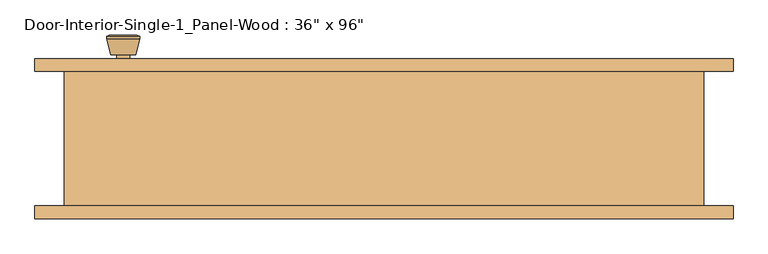
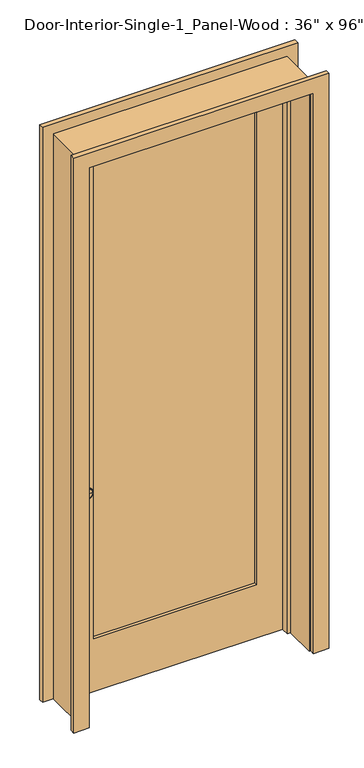
"""IFC4 building model written with IfcOpenShell, lengths in millimetres: door geometry."""

from ifc_helpers import new_model, si_unit, point, frame, frame_2d, origin, place, context, project, spatial, polyline, circle_curve, trimmed, segment, composite_curve, outline, extrude, faceted_brep, source, transform, mapped, element, save
from ifc_brep_helpers import plane_surface, cylinder_surface, revolved_surface, advanced_brep


def door_8805718f(model_context):
    return source(origin(), model_context, "Body", "SolidModel", [
        advanced_brep(
        [(-393.7, 57.5, 914.4), (-383.7, 57.5, 914.4), (-403.7, 57.5, 914.4), (-373.2241324, 8.5, 914.4), (-393.7, 8.5, 914.4), (-414.1758676, 8.5, 914.4), (-368.7, 10.3278681, 914.4), (-418.7, 10.3278681, 914.4), (-368.7, 13.7915463, 914.4), (-418.7, 13.7915463, 914.4), (-375.063764, 38.5, 914.4), (-412.336236, 38.5, 914.4), (-383.7, 38.5, 914.4), (-403.7, 38.5, 914.4)],
        [
            (0, 1),
            (1, 2, circle_curve(frame((-393.7, 57.5, 914.4), z_axis=(0.0, 1.0, 0.0), x_axis=(-1.0, 0.0, 0.0)), 10.0)),
            (2, 0),
            (2, 1, circle_curve(frame((-393.7, 57.5, 914.4), z_axis=(0.0, 1.0, 0.0), x_axis=(-1.0, 0.0, 0.0)), 10.0)),
            (3, 4),
            (4, 5),
            (5, 3, circle_curve(frame((-393.7, 8.5, 914.4), z_axis=(0.0, -1.0, 0.0), x_axis=(-1.0, 0.0, 0.0)), 20.4758676)),
            (3, 5, circle_curve(frame((-393.7, 8.5, 914.4), z_axis=(0.0, -1.0, 0.0), x_axis=(-1.0, 0.0, 0.0)), 20.4758676)),
            (6, 3),
            (5, 7),
            (7, 6, circle_curve(frame((-393.7, 10.3278681, 914.4), z_axis=(0.0, -1.0, 0.0), x_axis=(-1.0, 0.0, 0.0)), 25.0)),
            (6, 7, circle_curve(frame((-393.7, 10.3278681, 914.4), z_axis=(0.0, -1.0, 0.0), x_axis=(-1.0, 0.0, 0.0)), 25.0)),
            (8, 6),
            (7, 9),
            (9, 8, circle_curve(frame((-393.7, 13.7915463, 914.4), z_axis=(0.0, -1.0, 0.0), x_axis=(-1.0, 0.0, 0.0)), 25.0)),
            (8, 9, circle_curve(frame((-393.7, 13.7915463, 914.4), z_axis=(0.0, -1.0, 0.0), x_axis=(-1.0, 0.0, 0.0)), 25.0)),
            (10, 8),
            (9, 11),
            (11, 10, circle_curve(frame((-393.7, 38.5, 914.4), z_axis=(0.0, -1.0, 0.0), x_axis=(-1.0, 0.0, 0.0)), 18.636236)),
            (10, 11, circle_curve(frame((-393.7, 38.5, 914.4), z_axis=(0.0, -1.0, 0.0), x_axis=(-1.0, 0.0, 0.0)), 18.636236)),
            (12, 10),
            (11, 13),
            (13, 12, circle_curve(frame((-393.7, 38.5, 914.4), z_axis=(0.0, -1.0, 0.0), x_axis=(-1.0, 0.0, 0.0)), 10.0)),
            (12, 13, circle_curve(frame((-393.7, 38.5, 914.4), z_axis=(0.0, -1.0, 0.0), x_axis=(-1.0, 0.0, 0.0)), 10.0)),
            (1, 12),
            (13, 2),
        ],
        [
            plane_surface(frame((-393.7, 57.5, 914.4), z_axis=(0.0, 1.0, 0.0), x_axis=(-1.0, 0.0, 0.0))),
            plane_surface(frame((-393.7, 8.5, 914.4), z_axis=(0.0, -1.0, 0.0), x_axis=(-1.0, 0.0, 0.0))),
            revolved_surface(polyline([(-414.1758676, 8.5, 914.4), (-418.7, 10.3278681, 914.4)]), (-393.7, 57.5, 914.4), (0.0, 1.0, 0.0)),
            cylinder_surface(frame((-393.7, 57.5, 914.4), z_axis=(0.0, 1.0, 0.0), x_axis=(-1.0, 0.0, 0.0)), 25.0),
            revolved_surface(polyline([(-418.7, 13.7915463, 914.4), (-412.336236, 38.5, 914.4)]), (-393.7, 57.5, 914.4), (0.0, 1.0, 0.0)),
            plane_surface(frame((-393.7, 38.5, 914.4), z_axis=(0.0, 1.0, 0.0), x_axis=(-1.0, 0.0, 0.0))),
            cylinder_surface(frame((-393.7, 57.5, 914.4), z_axis=(0.0, 1.0, 0.0), x_axis=(-1.0, 0.0, 0.0)), 10.0),
        ],
        [
            (0, [[1, 2, 3]]),
            (0, [[-3, 4, -1]]),
            (1, [[5, 6, 7]]),
            (1, [[-6, -5, 8]]),
            (2, [[9, -7, 10, 11]]),
            (2, [[-10, -8, -9, 12]]),
            (3, [[13, -11, 14, 15]]),
            (3, [[-14, -12, -13, 16]]),
            (4, [[17, -15, 18, 19]]),
            (4, [[-18, -16, -17, 20]]),
            (5, [[21, -19, 22, 23]]),
            (5, [[-22, -20, -21, 24]]),
            (6, [[25, -23, 26, -2]]),
            (6, [[-26, -24, -25, -4]]),
        ],
    ),
        extrude(outline(composite_curve([segment(trimmed(circle_curve(frame_2d((914.4, -393.7)), 30.0), [point((914.4, -423.7))], [point((914.4, -363.7))], False, "CARTESIAN"), True, "CONTINUOUS"), segment(trimmed(circle_curve(frame_2d((914.4, -393.7)), 30.0), [point((914.4, -363.7))], [point((914.4, -423.7))], False, "CARTESIAN"), True, "CONTINUOUS")], self_intersect=False)), frame((0.0, 57.5, 0.0), z_axis=(0.0, 1.0, 0.0), x_axis=(0.0, 0.0, 1.0)), (0.0, 0.0, 1.0), 6.0),
        advanced_brep(
        [(-393.7, 104.425, 914.4), (-403.7, 104.425, 914.4), (-383.7, 104.425, 914.4), (-373.2241324, 153.425, 914.4), (-414.1758676, 153.425, 914.4), (-393.7, 153.425, 914.4), (-368.7, 151.5971319, 914.4), (-418.7, 151.5971319, 914.4), (-368.7, 148.1334537, 914.4), (-418.7, 148.1334537, 914.4), (-375.063764, 123.425, 914.4), (-412.336236, 123.425, 914.4), (-383.7, 123.425, 914.4), (-403.7, 123.425, 914.4)],
        [
            (0, 1),
            (1, 2, circle_curve(frame((-393.7, 104.425, 914.4), z_axis=(0.0, -1.0, 0.0), x_axis=(-1.0, 0.0, 0.0)), 10.0)),
            (2, 0),
            (2, 1, circle_curve(frame((-393.7, 104.425, 914.4), z_axis=(0.0, -1.0, 0.0), x_axis=(-1.0, 0.0, 0.0)), 10.0)),
            (3, 4, circle_curve(frame((-393.7, 153.425, 914.4), z_axis=(0.0, 1.0, 0.0), x_axis=(-1.0, 0.0, 0.0)), 20.4758676)),
            (4, 5),
            (5, 3),
            (4, 3, circle_curve(frame((-393.7, 153.425, 914.4), z_axis=(0.0, 1.0, 0.0), x_axis=(-1.0, 0.0, 0.0)), 20.4758676)),
            (6, 7, circle_curve(frame((-393.7, 151.5971319, 914.4), z_axis=(0.0, 1.0, 0.0), x_axis=(-1.0, 0.0, 0.0)), 25.0)),
            (7, 4),
            (3, 6),
            (7, 6, circle_curve(frame((-393.7, 151.5971319, 914.4), z_axis=(0.0, 1.0, 0.0), x_axis=(-1.0, 0.0, 0.0)), 25.0)),
            (8, 9, circle_curve(frame((-393.7, 148.1334537, 914.4), z_axis=(0.0, 1.0, 0.0), x_axis=(-1.0, 0.0, 0.0)), 25.0)),
            (9, 7),
            (6, 8),
            (9, 8, circle_curve(frame((-393.7, 148.1334537, 914.4), z_axis=(0.0, 1.0, 0.0), x_axis=(-1.0, 0.0, 0.0)), 25.0)),
            (10, 11, circle_curve(frame((-393.7, 123.425, 914.4), z_axis=(0.0, 1.0, 0.0), x_axis=(-1.0, 0.0, 0.0)), 18.636236)),
            (11, 9),
            (8, 10),
            (11, 10, circle_curve(frame((-393.7, 123.425, 914.4), z_axis=(0.0, 1.0, 0.0), x_axis=(-1.0, 0.0, 0.0)), 18.636236)),
            (12, 13, circle_curve(frame((-393.7, 123.425, 914.4), z_axis=(0.0, 1.0, 0.0), x_axis=(-1.0, 0.0, 0.0)), 10.0)),
            (13, 11),
            (10, 12),
            (13, 12, circle_curve(frame((-393.7, 123.425, 914.4), z_axis=(0.0, 1.0, 0.0), x_axis=(-1.0, 0.0, 0.0)), 10.0)),
            (1, 13),
            (12, 2),
        ],
        [
            plane_surface(frame((-393.7, 104.425, 914.4), z_axis=(0.0, -1.0, 0.0), x_axis=(-1.0, 0.0, 0.0))),
            plane_surface(frame((-393.7, 153.425, 914.4), z_axis=(0.0, 1.0, 0.0), x_axis=(-1.0, 0.0, 0.0))),
            revolved_surface(polyline([(-414.1758676, 153.425, 914.4), (-418.7, 151.5971319, 914.4)]), (-393.7, 104.425, 914.4), (0.0, -1.0, 0.0)),
            cylinder_surface(frame((-393.7, 104.425, 914.4), z_axis=(0.0, -1.0, 0.0), x_axis=(-1.0, 0.0, 0.0)), 25.0),
            revolved_surface(polyline([(-418.7, 148.1334537, 914.4), (-412.336236, 123.425, 914.4)]), (-393.7, 104.425, 914.4), (0.0, -1.0, 0.0)),
            plane_surface(frame((-393.7, 123.425, 914.4), z_axis=(0.0, -1.0, 0.0), x_axis=(-1.0, 0.0, 0.0))),
            cylinder_surface(frame((-393.7, 104.425, 914.4), z_axis=(0.0, -1.0, 0.0), x_axis=(-1.0, 0.0, 0.0)), 10.0),
        ],
        [
            (0, [[1, 2, 3]]),
            (0, [[-3, 4, -1]]),
            (1, [[5, 6, 7]]),
            (1, [[8, -7, -6]]),
            (2, [[9, 10, -5, 11]]),
            (2, [[12, -11, -8, -10]]),
            (3, [[13, 14, -9, 15]]),
            (3, [[16, -15, -12, -14]]),
            (4, [[17, 18, -13, 19]]),
            (4, [[20, -19, -16, -18]]),
            (5, [[21, 22, -17, 23]]),
            (5, [[24, -23, -20, -22]]),
            (6, [[-2, 25, -21, 26]]),
            (6, [[-4, -26, -24, -25]]),
        ],
    ),
        extrude(outline(composite_curve([segment(trimmed(circle_curve(frame_2d((914.4, -393.7)), 30.0), [point((914.4, -423.7))], [point((914.4, -363.7))], False, "CARTESIAN"), True, "CONTINUOUS"), segment(trimmed(circle_curve(frame_2d((914.4, -393.7)), 30.0), [point((914.4, -363.7))], [point((914.4, -423.7))], False, "CARTESIAN"), True, "CONTINUOUS")], self_intersect=False)), frame((0.0, 98.425, 0.0), z_axis=(0.0, 1.0, 0.0), x_axis=(0.0, 0.0, 1.0)), (0.0, 0.0, 1.0), 6.0),
        faceted_brep([(482.6, 98.425, 0.0), (482.6, -104.775, 0.0), (457.2, -104.775, 0.0), (457.2, 28.575, 0.0), (444.5, 28.575, 0.0), (444.5, 63.5, 0.0), (457.2, 63.5, 0.0), (457.2, 98.425, 0.0), (482.6, 98.425, 2463.8), (482.6, -104.775, 2463.8), (-482.6, -104.775, 2463.8), (-482.6, -104.775, 0.0), (-457.2, -104.775, 0.0), (-457.2, -104.775, 2438.4), (457.2, -104.775, 2438.4), (457.2, 28.575, 2438.4), (-457.2, 28.575, 2438.4), (-457.2, 28.575, 0.0), (-444.5, 28.575, 0.0), (-444.5, 28.575, 2425.7), (444.5, 28.575, 2425.7), (444.5, 63.5, 2425.7), (-444.5, 63.5, 2425.7), (-444.5, 63.5, 0.0), (-457.2, 63.5, 0.0), (-457.2, 63.5, 2438.4), (457.2, 63.5, 2438.4), (457.2, 98.425, 2438.4), (-457.2, 98.425, 2438.4), (-457.2, 98.425, 0.0), (-482.6, 98.425, 0.0), (-482.6, 98.425, 2463.8)], [[[0, 1, 2, 3, 4, 5, 6, 7]], [[1, 0, 8, 9]], [[2, 1, 9, 10, 11, 12, 13, 14]], [[3, 2, 14, 15]], [[4, 3, 15, 16, 17, 18, 19, 20]], [[5, 4, 20, 21]], [[6, 5, 21, 22, 23, 24, 25, 26]], [[7, 6, 26, 27]], [[0, 7, 27, 28, 29, 30, 31, 8]], [[9, 8, 31, 10]], [[15, 14, 13, 16]], [[21, 20, 19, 22]], [[27, 26, 25, 28]], [[30, 29, 24, 23, 18, 17, 12, 11]], [[10, 31, 30, 11]], [[16, 13, 12, 17]], [[22, 19, 18, 23]], [[28, 25, 24, 29]]]),
        extrude(outline(polyline([(2438.4, -457.2), (0.0, -457.2), (0.0, 457.2), (2438.4, 457.2), (2438.4, -457.2)]), holes=[polyline([(2319.3375, -336.55), (2319.3375, 336.55), (231.775, 336.55), (231.775, -336.55), (2319.3375, -336.55)])]), frame((0.0, 63.5, 0.0), z_axis=(0.0, 1.0, 0.0), x_axis=(0.0, 0.0, 1.0)), (0.0, 0.0, 1.0), 34.925),
        extrude(outline(polyline([(336.55, 75.1416667), (-336.55, 75.1416667), (-336.55, 86.7833333), (336.55, 86.7833333), (336.55, 75.1416667)])), frame((0.0, 0.0, 231.775), z_axis=(0.0, 0.0, 1.0), x_axis=(1.0, 0.0, 0.0)), (0.0, 0.0, 1.0), 2087.5625),
        extrude(outline(polyline([(0.0, 463.55), (0.0, 527.05), (2508.25, 527.05), (2508.25, -527.05), (0.0, -527.05), (0.0, -463.55), (2444.75, -463.55), (2444.75, 463.55), (0.0, 463.55)])), frame((0.0, 98.425, 0.0), z_axis=(0.0, 1.0, 0.0), x_axis=(0.0, 0.0, 1.0)), (0.0, 0.0, 1.0), 19.05),
        extrude(outline(polyline([(0.0, 463.55), (0.0, 527.05), (2508.25, 527.05), (2508.25, -527.05), (0.0, -527.05), (0.0, -463.55), (2444.75, -463.55), (2444.75, 463.55), (0.0, 463.55)])), frame((0.0, -123.825, 0.0), z_axis=(0.0, 1.0, 0.0), x_axis=(0.0, 0.0, 1.0)), (0.0, 0.0, 1.0), 19.05),
    ])


if __name__ == "__main__":
    model = new_model("IFC4")
    model_context = context("Model", 3, world=origin())
    ifc_project = project(units=[si_unit("LENGTHUNIT", "METRE", prefix="MILLI")], contexts=[model_context])
    site = spatial("IfcSite", under=ifc_project)
    building = spatial("IfcBuilding", under=site)
    placement = place(None, origin())
    door_shape = door_8805718f(model_context)
    element("IfcDoor", 1, ObjectType="Door-Interior-Single-1_Panel-Wood : 36\" x 96\"", at=placement, inside=building, context=model_context, shape_type="MappedRepresentation", body=[
        mapped(door_shape, transform((0.0, 0.0, 0.0), x_axis=(1.0, 0.0, 0.0), y_axis=(0.0, 1.0, 0.0), z_axis=(0.0, 0.0, 1.0))),
    ])
    save(model, "model.ifc")

# Revit data of these elements
# Type "Door-Interior-Single-1_Panel-Wood : 36\" x 96\""
#   Type Mark = "8"
#   Assembly Code = "C1020300"
#   Analytic Construction = "Wooden"
#   Top Rail = 0' - 4 11/16"
#   Thickness = 0' - 1 3/8"
#   Thermal Resistance (R) = 2.5876 (h·ft²·°F)/BTU
#   Swing Angle [instance default] = 90.00°
#   Stiles = 0' - 4 3/4"
#   Rough Width = 3' - 2"
#   Rough Height = 8' - 1"
#   Height = 8' - 0"
#   Width = 3' - 0"
#   Heat Transfer Coefficient (U) = 0.3865 BTU/(h·ft²·°F)
#   Bottom Rail = 0' - 9 1/8"
#   Trim Material = Cherry
#   Panel Material = Cherry
#   Frame Material = Cherry
#   Door Handle Material = Aluminum
#   Visual Light Transmittance = 0
#   Solar Heat Gain Coefficient = 0
#   Wall Closure = (empty or 0)
#   Function = (empty or 0)
# Element 1 (IfcDoor, "Door-Interior-Single-1_Panel-Wood : 36\" x 96\"")
#   Materials on its faces: "Cherry", "Aluminum"
# Materials
#   "Cherry": class "Wood", colour RGB 226 177 128, transparency 0, Description = "Prunus Serotina", Cost = 0
#   "Aluminum": class "Metal", colour RGB 247 247 247, transparency 0, Description = "Aluminum 6061", Cost = 0
